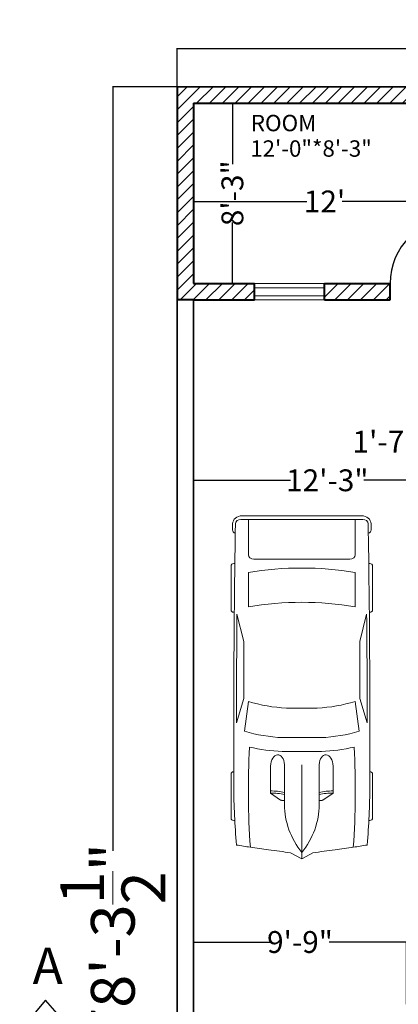
# Model space of a CAD drawing. Units: inches. Extents: x 1146 to 2917, y 889 to 2437.
# Tile 5 of 13: x 1219 to 1427, y 1867 to 2408. Entities that reach past the tile are written whole.
import ezdxf

# ---------------------------------------------------------------- set-up
doc = ezdxf.new("R2010")
doc.units = ezdxf.units.IN
doc.header["$MEASUREMENT"] = 0
for name, color, linetype, lineweight in [('A-ANNO-DIMS', 2, 'Continuous', 18), ('A-ANNO-SYMB', 7, 'Continuous', 25), ('A-AREA-IDEN', 7, 'Continuous', 18), ('A-SITE-VEHC', 8, 'Continuous', 13), ('A-SITE-WALL', 7, 'Continuous', 35), ('A-WALL-PATT', 163, 'Continuous', 13), ('door', 10, 'Continuous', 25), ('wall', 7, 'Continuous', 40), ('window', 5, 'Continuous', 18)]:
    doc.layers.add(name, color=color, linetype=linetype, lineweight=lineweight)
doc.styles.get("Standard").update_dxf_attribs({"font": 'arial.ttf'})
doc.dimstyles.new('Copy of Standard', dxfattribs={"dimtxt": 24, "dimasz": 0.18, "dimexe": 0.18, "dimexo": 0.0625, "dimgap": 0.09, "dimtad": 0, "dimtoh": 1, "dimdec": 1, "dimzin": 0, "dimdsep": 46, "dimlunit": 4, "dimtxsty": 'Standard', "dimcen": 0.09, "dimadec": 0, "dimazin": 0, "dimtfac": 1, "dimtdec": 1, "dimtofl": 0, "dimtmove": 0, "dimatfit": 3, "dimfxl": 1, "dimtolj": 1, "dimtzin": 0, "dimarcsym": 0})
doc.dimstyles.get("Standard").update_dxf_attribs({"dimtxt": 12, "dimasz": 0.18, "dimexe": 0.18, "dimexo": 0.0625, "dimgap": 0.09, "dimtad": 0, "dimtoh": 1, "dimdec": 1, "dimzin": 0, "dimdsep": 46, "dimlunit": 4, "dimtxsty": 'Standard', "dimcen": 0.09, "dimadec": 0, "dimazin": 0, "dimtfac": 1, "dimtdec": 1, "dimtofl": 0, "dimtmove": 0, "dimatfit": 3, "dimfxl": 1, "dimtolj": 1, "dimtzin": 0, "dimarcsym": 0})

# ---------------------------------------------------------------- blocks, each defined once
blk = doc.blocks.new('*D1')
at = {"layer": 'A-ANNO-DIMS', "color": 0, "lineweight": -2, "transparency": 16777216}
for p, q in [((1314.13, 2182.33), (1314.13, 2155.05)), ((1461.13, 2182.33), (1461.13, 2155.05)), ((1314.31, 2155.23), (1367.5, 2155.23)), ((1460.95, 2155.23), (1407.77, 2155.23))]:
    blk.add_line(p, q, dxfattribs=at)
at = {"layer": 'A-ANNO-DIMS', "color": 0, "transparency": 16777216}
for points in [[(1314.31, 2155.26), (1314.31, 2155.2), (1314.13, 2155.23)], [(1460.95, 2155.26), (1460.95, 2155.2), (1461.13, 2155.23)]]:
    blk.add_solid(points, dxfattribs=at)
at = {"layer": 'Defpoints', "color": 0, "transparency": 16777216}
for p in [(1314.13, 2182.39), (1461.13, 2182.39), (1314.13, 2155.23)]:
    blk.add_point(p, dxfattribs=at)
at = {"layer": 'A-ANNO-DIMS', "color": 0, "transparency": 16777216, "insert": (1387.63, 2155.23), "char_height": 12, "attachment_point": 5}
blk.add_mtext('\\A1;12\'-3"', dxfattribs=at)
blk = doc.blocks.new('*D6')
at = {"layer": 'A-ANNO-DIMS', "color": 0, "lineweight": -2, "transparency": 16777216}
for p, q in [((1314.13, 2362.33), (1314.13, 2308.21)), ((1458.13, 2362.33), (1458.13, 2308.21)), ((1314.31, 2308.39), (1376.43, 2308.39)), ((1457.95, 2308.39), (1395.84, 2308.39))]:
    blk.add_line(p, q, dxfattribs=at)
at = {"layer": 'A-ANNO-DIMS', "color": 0, "transparency": 16777216}
for points in [[(1314.31, 2308.42), (1314.31, 2308.36), (1314.13, 2308.39)], [(1457.95, 2308.42), (1457.95, 2308.36), (1458.13, 2308.39)]]:
    blk.add_solid(points, dxfattribs=at)
at = {"layer": 'Defpoints', "color": 0, "transparency": 16777216}
for p in [(1314.13, 2362.39), (1458.13, 2362.39), (1458.13, 2308.39)]:
    blk.add_point(p, dxfattribs=at)
at = {"layer": 'A-ANNO-DIMS', "color": 0, "transparency": 16777216, "insert": (1386.13, 2308.39), "char_height": 12, "attachment_point": 5}
blk.add_mtext("\\A1;12'", dxfattribs=at)
blk = doc.blocks.new('*U18')
for p, q in [((-24, 0), (-24, -6)), ((0, 0), (0, -6))]:
    blk.add_line(p, q)
blk.add_lwpolyline([(0, 0), (0, 24), (-1.75, 24), (-1.75, 0)], close=True)
blk.add_arc((0, 0), 24, 90, 180)
blk = doc.blocks.new('*D49')
at = {"layer": 'A-ANNO-DIMS', "color": 0, "lineweight": -2, "transparency": 16777216}
for p, q in [((1314.13, 1867.45), (1314.13, 1901.79)), ((1314.31, 1901.61), (1356.59, 1901.61)), ((1430.95, 1901.61), (1388.67, 1901.61)), ((1431.13, 1867.45), (1431.13, 1901.79))]:
    blk.add_line(p, q, dxfattribs=at)
at = {"layer": 'A-ANNO-DIMS', "color": 0, "transparency": 16777216}
for points in [[(1314.31, 1901.64), (1314.31, 1901.58), (1314.13, 1901.61)], [(1430.95, 1901.64), (1430.95, 1901.58), (1431.13, 1901.61)]]:
    blk.add_solid(points, dxfattribs=at)
at = {"layer": 'Defpoints', "color": 0, "transparency": 16777216}
for p in [(1314.13, 1901.61), (1314.13, 1867.39), (1431.13, 1867.39)]:
    blk.add_point(p, dxfattribs=at)
at = {"layer": 'A-ANNO-DIMS', "color": 0, "transparency": 16777216, "insert": (1372.63, 1901.61), "char_height": 12, "attachment_point": 5}
blk.add_mtext('\\A1;9\'-9"', dxfattribs=at)
blk = doc.blocks.new('*D52')
at = {"layer": 'A-ANNO-DIMS', "color": 0, "lineweight": -2, "transparency": 16777216}
for p, q in [((1314.2, 2362.39), (1335.69, 2362.39)), ((1335.51, 2362.21), (1335.51, 2328.94)), ((1335.51, 2263.57), (1335.51, 2296.84)), ((1314.2, 2263.39), (1335.69, 2263.39))]:
    blk.add_line(p, q, dxfattribs=at)
at = {"layer": 'A-ANNO-DIMS', "color": 0, "transparency": 16777216}
for points in [[(1335.48, 2362.21), (1335.54, 2362.21), (1335.51, 2362.39)], [(1335.48, 2263.57), (1335.54, 2263.57), (1335.51, 2263.39)]]:
    blk.add_solid(points, dxfattribs=at)
at = {"layer": 'Defpoints', "color": 0, "transparency": 16777216}
for p in [(1314.13, 2362.39), (1314.13, 2263.39), (1335.51, 2263.39)]:
    blk.add_point(p, dxfattribs=at)
at = {"layer": 'A-ANNO-DIMS', "color": 0, "transparency": 16777216, "insert": (1335.51, 2312.89), "char_height": 12, "attachment_point": 5, "rotation": 90}
blk.add_mtext('\\A1;8\'-3"', dxfattribs=at)
blk = doc.blocks.new('*D53')
at = {"layer": 'A-ANNO-DIMS', "color": 0, "lineweight": -2, "transparency": 16777216}
for p, q in [((1305.13, 2371.45), (1305.13, 2392.67)), ((1305.31, 2392.49), (1616.32, 2392.49)), ((2009.95, 2392.49), (1698.95, 2392.49)), ((2010.13, 2371.45), (2010.13, 2392.67))]:
    blk.add_line(p, q, dxfattribs=at)
at = {"layer": 'A-ANNO-DIMS', "color": 0, "transparency": 16777216}
for points in [[(1305.31, 2392.52), (1305.31, 2392.46), (1305.13, 2392.49)], [(2009.95, 2392.52), (2009.95, 2392.46), (2010.13, 2392.49)]]:
    blk.add_solid(points, dxfattribs=at)
at = {"layer": 'Defpoints', "color": 0, "transparency": 16777216}
for p in [(2010.13, 2392.49), (1305.13, 2371.39), (2010.13, 2371.39)]:
    blk.add_point(p, dxfattribs=at)
at = {"layer": 'A-ANNO-DIMS', "color": 0, "transparency": 16777216, "insert": (1657.63, 2392.49), "char_height": 24, "attachment_point": 5}
blk.add_mtext('\\A1;58\'-9"', dxfattribs=at)
blk = doc.blocks.new('*D54')
at = {"layer": 'A-ANNO-DIMS', "color": 0, "lineweight": -2, "transparency": 16777216}
for p, q in [((1305.07, 2371.39), (1269.65, 2371.39)), ((1269.83, 2371.21), (1269.83, 1951.61)), ((1269.83, 1432.07), (1269.83, 1851.68)), ((1305.07, 1431.89), (1269.65, 1431.89))]:
    blk.add_line(p, q, dxfattribs=at)
at = {"layer": 'A-ANNO-DIMS', "color": 0, "transparency": 16777216}
for points in [[(1269.8, 2371.21), (1269.86, 2371.21), (1269.83, 2371.39)], [(1269.8, 1432.07), (1269.86, 1432.07), (1269.83, 1431.89)]]:
    blk.add_solid(points, dxfattribs=at)
at = {"layer": 'Defpoints', "color": 0, "transparency": 16777216}
for p in [(1305.13, 2371.39), (1269.83, 1431.89), (1305.13, 1431.89)]:
    blk.add_point(p, dxfattribs=at)
at = {"layer": 'A-ANNO-DIMS', "color": 0, "transparency": 16777216, "insert": (1269.83, 1901.64), "char_height": 24, "attachment_point": 5, "rotation": 90}
blk.add_mtext('\\A1;78\'-3{\\H1x;\\S1/2;}"', dxfattribs=at)
blk = doc.blocks.new('*U57')
for p, q in [((46.55, 38.89), (22.35, 38.89)), ((136.7, 38.89), (160.9, 38.89)), ((21.1, 37.41), (21.1, 36.83)), ((47.8, 37.39), (47.8, 37.41)), ((87.99, 31.87), (74.76, 35.92)), ((134.31, 35.6), (119.29, 31.78)), ((135.45, 37.07), (135.45, 37.41)), ((162.15, 37.41), (162.15, 36.77)), ((186.47, -33.5), (186.47, 33.5)), ((188.4, -32.76), (188.4, 32.76)), ((70.03, 31.54), (86.41, 29.35)), ((138.42, 29.35), (157.25, 29.35)), ((186.47, 29.35), (167.01, 29.35)), ((164.52, 26.39), (164.52, -26.39)), ((32.27, 11.63), (36.13, 17.17)), ((36.13, 17.17), (50.94, 17.17)), ((32.12, 9.51), (32.12, 11.15)), ((3.27, 6.13), (0.1, 0.41)), ((29.77, 9.51), (51.68, 9.51)), ((58.92, -10.77), (58.92, 10.77)), ((66.55, -10.53), (66.55, 10.53)), ((82.74, 8.5), (82.74, -8.5)), ((186.47, -10.53), (186.47, 10.53)), ((0, 0), (51.68, 0)), ((0.1, -0.41), (3.27, -6.13)), ((29.77, -9.51), (51.68, -9.51)), ((32.12, -9.51), (32.12, -11.15)), ((32.27, -11.63), (36.13, -17.17)), ((36.13, -17.17), (50.94, -17.17)), ((86.41, -29.35), (70.03, -31.54)), ((87.99, -31.87), (74.76, -35.92)), ((134.31, -35.6), (119.29, -31.78)), ((157.25, -29.35), (138.42, -29.35)), ((167.01, -29.35), (186.47, -29.35)), ((21.1, -37.41), (21.1, -36.83)), ((47.8, -37.39), (47.8, -37.41)), ((135.45, -37.07), (135.45, -37.41)), ((162.15, -37.41), (162.15, -36.77)), ((46.55, -38.89), (22.35, -38.89)), ((136.7, -38.89), (160.9, -38.89))]:
    blk.add_line(p, q)
for centre, major_axis, ratio, start_param, end_param in [((22.35, 37.41), (0, -1.48), 0.842304, 3.141593, 4.712389), ((46.55, 37.41), (0, 1.48), 0.842304, -1.570796, 0), ((136.7, 37.41), (0, -1.48), 0.842304, 3.141593, 4.712389), ((160.9, 37.41), (0, 1.48), 0.842304, -1.570796, 0), ((180.63, 35.84), (0, 2.22), 0.842304, -0.013017, 1.249894), ((64.48, -10556.36), (0, 10595.31), 0.842304, -0.013397, -0.013017), ((183.98, 32.76), (0, -5.25), 0.842304, 1.570796, 3.128196), ((266.03, -27.52), (0, 313.31), 0.842304, 1.367076, 1.39176), ((41.19, -490.86), (0, 528.23), 0.842304, 0.00281, 0.075598), ((64.48, -10555.62), (0, 10593.03), 0.842304, -0.013397, 0.002797), ((64.48, -10555.62), (0, -10591.55), 0.842304, 3.133765, 3.140441), ((183.98, 33.5), (0, -2.96), 0.842304, 1.570796, 3.128196), ((259.18, -27.52), (0, -305.3), 0.842304, 4.528606, 4.561838), ((37.47, -593.96), (0, -623.33), 0.842304, 3.096046, 3.200911), ((134.4, 5.39), (0, -89.78), 0.842304, 4.449482, 4.652344), ((135.29, 5.39), (0, 81.77), 0.842304, 1.245306, 1.50788), ((149.6, 2.8), (0, -79.58), 0.842304, 4.372215, 4.640744), ((95.79, -3666.35), (0, -3698.24), 0.842304, 3.134049, 3.144098), ((17.08, 0), (0, 147.02), 0.842304, 4.511394, 4.913384), ((35.91, 0), (0, 147.02), 0.842304, 4.511394, 4.913384), ((167.01, 26.39), (0, 2.96), 0.842304, 0, 1.570796), ((-204.49, 52.4), (0, -250.96), 0.842304, 1.385369, 1.434372), ((13.04, 17.01), (0, 27.42), 0.842304, 4.435146, 4.718221), ((14.2, 17.01), (0, 27.42), 0.842304, 4.435146, 4.718221), ((50.79, 13.34), (6.34, -0.36), 0.603834, -1.395552, 1.581315), ((32.75, 11.15), (0, 0.74), 0.842304, 0.879714, 1.570796), ((29.77, -46.66), (0, 56.17), 0.842304, 0, 0.590319), ((0.62, 0), (0, -0.74), 0.842304, 4.131459, 5.293319), ((29.77, 46.66), (0, 56.17), 0.842304, 2.551274, 3.141593), ((-204.49, -52.4), (0, 250.96), 0.842304, -1.434372, -1.385369), ((13.04, -17.01), (0, -27.42), 0.842304, 1.564964, 1.848039), ((14.2, -17.01), (0, -27.42), 0.842304, 1.564964, 1.848039), ((134.4, -5.39), (0, -89.78), 0.842304, -1.510751, -1.307889), ((135.29, -5.39), (0, -81.77), 0.842304, -1.50788, -1.245306), ((149.6, -2.8), (0, -79.58), 0.842304, -1.499151, -1.230623), ((32.75, -11.15), (0, -0.74), 0.842304, 4.712389, 5.403472), ((259.18, 27.52), (0, 305.3), 0.842304, 1.721348, 1.754579), ((167.01, -26.39), (0, -2.96), 0.842304, 4.712389, 6.283185), ((266.03, 27.52), (0, 313.31), 0.842304, 1.749832, 1.774517), ((37.47, 593.96), (0, -623.33), 0.842304, -0.059319, 0.045547), ((95.79, 3666.35), (0, -3698.24), 0.842304, -0.002505, 0.007544), ((41.19, 490.86), (0, -528.23), 0.842304, -0.075598, -0.00281), ((22.35, -37.41), (0, 1.48), 0.842304, 1.570796, 3.141593), ((64.48, 10555.62), (0, 10593.03), 0.842304, 3.138796, 3.15499), ((46.55, -37.41), (0, -1.48), 0.842304, 0, 1.570796), ((64.48, 10555.62), (0, -10591.55), 0.842304, 0.001152, 0.007828), ((136.7, -37.41), (0, -1.48), 0.842304, -1.570796, 0), ((160.9, -37.41), (0, 1.48), 0.842304, 3.141593, 4.712389), ((180.63, -35.84), (0, -2.22), 0.842304, -1.249894, 0.013017), ((183.98, -33.5), (0, 2.96), 0.842304, 3.15499, 4.712389), ((183.98, -32.76), (0, -5.25), 0.842304, 0.013397, 1.570796), ((64.48, 10556.36), (0, 10595.31), 0.842304, 3.15461, 3.15499)]:
    blk.add_ellipse(centre, major_axis=major_axis, ratio=ratio, start_param=start_param, end_param=end_param)
at = {"extrusion": (0, 0, -1)}
blk.add_ellipse((50.79, -13.34), major_axis=(6.34, 0.36), ratio=0.603834, start_param=-1.395552, end_param=1.581315, dxfattribs=at)
blk = doc.blocks.new('SECTION-HEAD')
for p, q in [((14.15, 39.3), (0, 22.6)), ((28.83, 22.6), (14.15, 39.3)), ((0, 22.6), (28.83, 22.6)), ((14.15, 0), (14.15, 17.21))]:
    blk.add_line(p, q)
blk.add_arc((14.15, 26.98), 9.77, 206.6471, 333.3529)
blk = doc.blocks.new('*D100')
at = {"layer": 'A-ANNO-DIMS', "color": 0, "lineweight": -2, "transparency": 16777216}
for p, q in [((1502.51, 2176.45), (1502.33, 2176.45)), ((1502.51, 2173.45), (1502.51, 2176.63)), ((1521.6, 2176.45), (1502.69, 2176.45)), ((1521.78, 2173.45), (1521.78, 2176.63))]:
    blk.add_line(p, q, dxfattribs=at)
at = {"layer": 'A-ANNO-DIMS', "color": 0, "transparency": 16777216}
for points in [[(1502.69, 2176.48), (1502.69, 2176.42), (1502.51, 2176.45)], [(1521.6, 2176.48), (1521.6, 2176.42), (1521.78, 2176.45)]]:
    blk.add_solid(points, dxfattribs=at)
at = {"layer": 'Defpoints', "color": 0, "transparency": 16777216}
for p in [(1502.51, 2176.45), (1502.51, 2173.39), (1521.78, 2173.39)]:
    blk.add_point(p, dxfattribs=at)
at = {"layer": 'A-ANNO-DIMS', "color": 0, "transparency": 16777216, "insert": (1452.25, 2176.45), "char_height": 12, "attachment_point": 5}
blk.add_mtext('\\A1;1\'-7 1/2" TYP.', dxfattribs=at)

msp = doc.modelspace()

# ---------------------------------------------------------------- hatches: boundary and pattern name
at = {"layer": 'A-WALL-PATT'}
h = msp.add_hatch(dxfattribs=at)
h.set_pattern_fill('ANSI31', color=256, scale=40)
h.paths.add_polyline_path([(1773.13, 2371.39), (1305.13, 2371.39), (1305.13, 2362.39), (1305.13, 2254.39), (1314.13, 2254.39), (1347.63, 2254.39), (1347.63, 2263.39), (1314.13, 2263.39), (1314.13, 2362.39), (1458.13, 2362.39), (1458.13, 2254.39), (1467.13, 2254.39), (1500.63, 2254.39), (1500.63, 2263.39), (1467.13, 2263.39), (1467.13, 2362.39), (1611.13, 2362.39), (1611.13, 2254.39), (1620.13, 2254.39), (1620.13, 2362.39), (1764.13, 2362.39), (1764.13, 2263.39), (1730.63, 2263.39), (1730.63, 2254.39), (1773.13, 2254.39), (1773.13, 2362.39)])
h.paths.add_polyline_path([(1422.13, 2263.39), (1386.13, 2263.39), (1386.13, 2254.39), (1422.13, 2254.39)], flags=17)
h.paths.add_polyline_path([(1575.13, 2263.39), (1539.13, 2263.39), (1539.13, 2254.39), (1575.13, 2254.39)], flags=17)
h.paths.add_polyline_path([(1692.13, 2263.39), (1656.13, 2263.39), (1656.13, 2254.39), (1692.13, 2254.39)], flags=17)

# ---------------------------------------------------------------- linework, layer by layer
at = {"layer": 'A-SITE-WALL'}
for p, q in [((1305.13, 2371.39), (2010.13, 2371.39)), ((1305.13, 2254.39), (1305.13, 1431.89)), ((1314.13, 2254.39), (1314.13, 1440.89))]:
    msp.add_line(p, q, dxfattribs=at)
at = {"layer": 'wall'}
for p, q in [((1305.13, 2371.39), (1305.13, 2362.39)), ((1305.13, 2362.39), (1305.13, 2254.39)), ((1314.13, 2362.39), (1458.13, 2362.39)), ((1314.13, 2362.39), (1314.13, 2263.39)), ((1314.13, 2263.39), (1347.63, 2263.39)), ((1347.63, 2254.39), (1347.63, 2263.39)), ((1386.13, 2254.39), (1386.13, 2263.39)), ((1386.13, 2263.39), (1422.13, 2263.39)), ((1422.13, 2254.39), (1422.13, 2263.39)), ((1314.13, 2254.39), (1305.13, 2254.39)), ((1314.13, 2254.39), (1347.63, 2254.39)), ((1386.13, 2254.39), (1422.13, 2254.39))]:
    msp.add_line(p, q, dxfattribs=at)
at = {"layer": 'window'}
for points in [[(1347.63, 2263.39), (1386.13, 2263.39), (1386.13, 2254.39), (1347.63, 2254.39)], [(1347.63, 2260.88), (1386.13, 2260.88), (1386.13, 2256.47), (1347.63, 2256.47)]]:
    msp.add_lwpolyline(points, close=True, dxfattribs=at)

# ---------------------------------------------------------------- block references
at = {"layer": 'A-ANNO-SYMB'}
msp.add_blockref('SECTION-HEAD', (1218.69, 1830.35), dxfattribs=at)
at = {"layer": 'A-SITE-VEHC', "rotation": 90}
msp.add_blockref('*U57', (1373.64, 1947.31), dxfattribs=at)
at = {"layer": 'door', "xscale": 1.500000000000009, "yscale": 1.500000000000009, "zscale": 1.500000000000009}
msp.add_blockref('*U18', (1458.13, 2263.39), dxfattribs=at)

# ---------------------------------------------------------------- texts
at = {"layer": 'A-ANNO-SYMB', "insert": (1225.78, 1898.56), "char_height": 20, "attachment_point": 1}
msp.add_mtext_dynamic_manual_height_columns('A', width=22.084, gutter_width=1, heights=[0], dxfattribs=at)
at = {"layer": 'A-AREA-IDEN', "char_height": 9, "attachment_point": 1}
for s, width, insert in [('ROOM', 65.2952, (1345.62, 2355.97)), ('12\'-0"*8\'-3"', 53.2403, (1345.3, 2341.97))]:
    msp.add_mtext_dynamic_manual_height_columns(s, width=width, gutter_width=1, heights=[0], dxfattribs=dict(at, insert=insert))

# ---------------------------------------------------------------- dimensions: what is measured, and where the dimension line sits
at = {"layer": 'A-ANNO-DIMS'}
for p1, p2, distance, dimstyle, picture, middle in [((1305.13, 2371.39), (2010.13, 2371.39), 21.1, 'Copy of Standard', '*D53', (1657.63, 2392.49)), ((1314.13, 2362.39), (1458.13, 2362.39), -54, 'Standard', '*D6', (1386.13, 2308.39)), ((1314.13, 2362.39), (1314.13, 2263.39), 21.38, 'Standard', '*D52', (1335.51, 2312.89)), ((1461.13, 2182.39), (1314.13, 2182.39), 27.16, 'Standard', '*D1', (1387.63, 2155.23)), ((1431.13, 1867.39), (1314.13, 1867.39), -34.21, 'Standard', '*D49', (1372.63, 1901.61))]:
    dim = msp.add_aligned_dim(p1=p1, p2=p2, distance=distance, dimstyle=dimstyle, override={"dimclrd": 0, "dimclre": 0, "dimclrt": 0}, dxfattribs=at)
    dim.commit()
    dim.dimension.update_dxf_attribs({"geometry": picture, "text_midpoint": middle})
dim = msp.add_linear_dim(base=(1269.83, 1431.89), p1=(1305.13, 2371.39), p2=(1305.13, 1431.89), angle=270, dimstyle='Copy of Standard', override={"dimclrd": 0, "dimclre": 0, "dimclrt": 0}, dxfattribs=at)
dim.commit()
dim.dimension.update_dxf_attribs({"geometry": '*D54', "text_midpoint": (1269.83, 1901.64), "dimtype": 161})
dim = msp.add_linear_dim(base=(1502.51, 2176.45), p1=(1521.78, 2173.39), p2=(1502.51, 2173.39), angle=180, text='<> TYP.', dimstyle='Standard', override={"dimdec": 1, "dimlfac": 1, "dimrnd": 0, "dimzin": 1, "dimdsep": 46, "dimlunit": 4, "dimfrac": 2}, dxfattribs=at)
dim.commit()
dim.dimension.update_dxf_attribs({"geometry": '*D100', "text_midpoint": (1452.25, 2176.45)})

doc.saveas('drawing.dxf')
